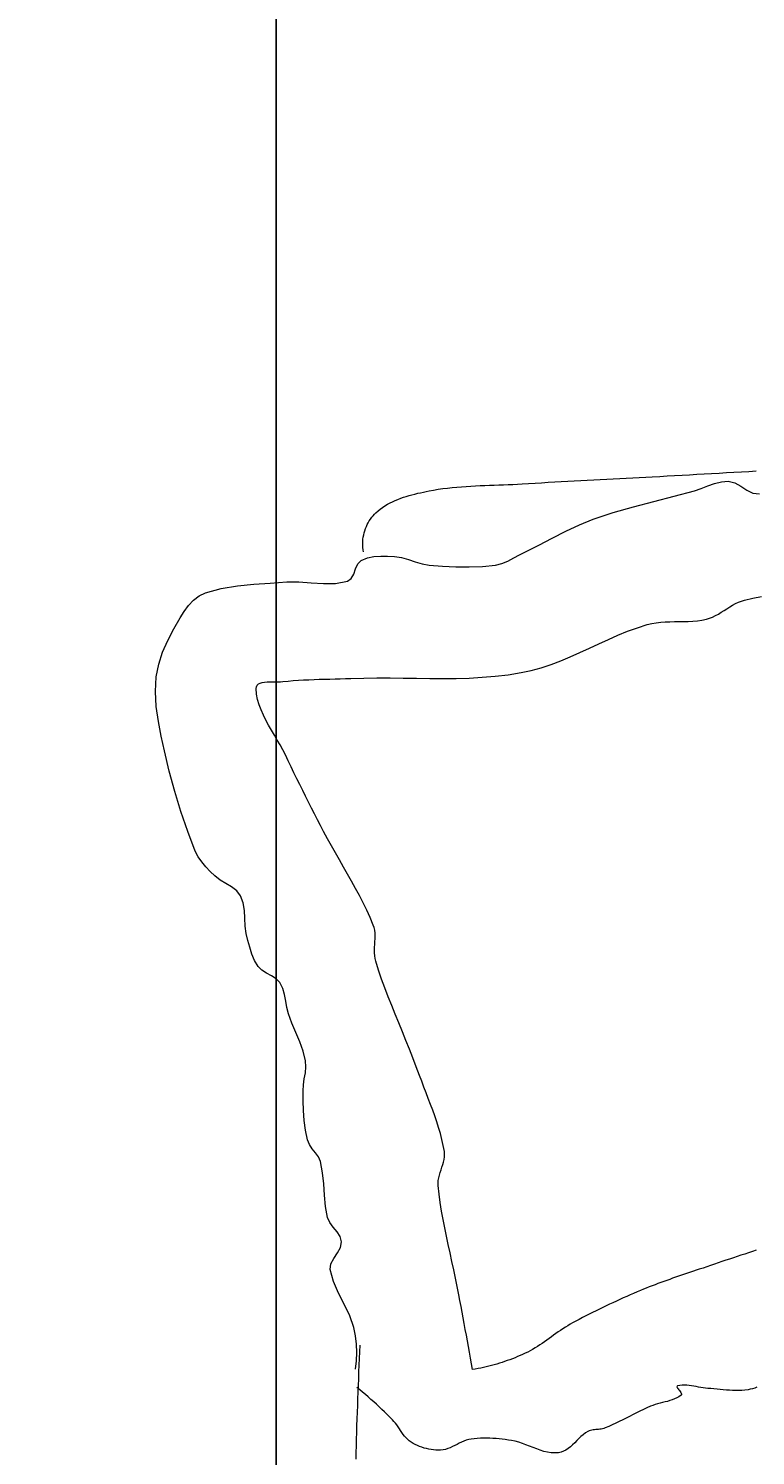
# Model space of a CAD drawing. Units: inches. Extents: x 1770 to 2988, y 1161 to 3221.
# Tile 26 of 44: x 2524 to 2543, y 2330 to 2368. Entities that reach past the tile are written whole.
import ezdxf

# ---------------------------------------------------------------- set-up
doc = ezdxf.new("R2010")
doc.units = ezdxf.units.IN
doc.layers.add('A-ANNO-DIMS', color=2, linetype='Continuous', lineweight=18)
doc.layers.add('A-FURN', color=8, linetype='Continuous', lineweight=13)
doc.styles.get("Standard").update_dxf_attribs({"font": 'arial.ttf'})
doc.dimstyles.get("Standard").update_dxf_attribs({"dimtxt": 0.18, "dimasz": 0.18, "dimexe": 0.18, "dimexo": 0.0625, "dimgap": 0.09, "dimtad": 0, "dimtih": 1, "dimtoh": 1, "dimdec": 4, "dimzin": 0, "dimdsep": 46, "dimtxsty": 'Standard', "dimcen": 0.09, "dimadec": 0, "dimazin": 0, "dimtfac": 1, "dimtdec": 4, "dimtofl": 0, "dimtmove": 0, "dimatfit": 3, "dimfxl": 1, "dimtolj": 1, "dimtzin": 0, "dimarcsym": 0})

# ---------------------------------------------------------------- blocks, each defined once
blk = doc.blocks.new('BED-DOUBLE-PLAN')
for p, q in [((10.769, 99.878), (10.891, 99.883)), ((10.891, 99.883), (11.012, 99.89)), ((11.012, 99.89), (11.134, 99.897)), ((11.134, 99.897), (11.304, 99.907)), ((11.304, 99.907), (11.474, 99.918)), ((11.474, 99.918), (11.644, 99.928)), ((11.644, 99.928), (11.814, 99.938)), ((11.814, 99.938), (11.984, 99.947)), ((11.984, 99.947), (12.154, 99.957)), ((12.154, 99.957), (12.324, 99.966)), ((12.324, 99.966), (12.493, 99.975)), ((12.493, 99.975), (12.663, 99.984)), ((12.663, 99.984), (12.833, 99.993)), ((12.833, 99.993), (13.003, 100.002)), ((13.003, 100.002), (13.173, 100.011)), ((13.173, 100.011), (13.343, 100.019)), ((13.343, 100.019), (13.513, 100.028)), ((13.513, 100.028), (13.683, 100.037)), ((13.683, 100.037), (13.853, 100.046)), ((13.853, 100.046), (14.023, 100.055)), ((14.023, 100.055), (14.193, 100.064)), ((14.193, 100.064), (14.363, 100.073)), ((14.363, 100.073), (14.533, 100.083)), ((14.533, 100.083), (14.727, 100.093)), ((14.727, 100.093), (14.92, 100.104)), ((14.92, 100.104), (15.114, 100.115)), ((15.114, 100.115), (15.308, 100.126)), ((15.308, 100.126), (15.501, 100.137)), ((15.501, 100.137), (15.695, 100.147)), ((15.695, 100.147), (15.888, 100.158)), ((15.888, 100.158), (16.082, 100.169)), ((15.984, 99.845), (16.159, 99.909)), ((16.082, 100.169), (16.276, 100.18)), ((16.159, 99.909), (16.336, 99.954)), ((16.276, 100.18), (16.469, 100.191)), ((16.336, 99.954), (16.516, 99.966)), ((16.469, 100.191), (16.663, 100.202)), ((16.516, 99.966), (16.685, 99.923)), ((16.663, 100.202), (16.857, 100.213)), ((16.685, 99.923), (16.844, 99.835)), ((16.857, 100.213), (17.05, 100.224)), ((17.05, 100.224), (17.244, 100.235)), ((7.892, 99.493), (7.964, 99.52)), ((7.964, 99.52), (8.036, 99.546)), ((8.036, 99.546), (8.109, 99.569)), ((8.109, 99.569), (8.183, 99.591)), ((8.183, 99.591), (8.258, 99.612)), ((8.258, 99.612), (8.332, 99.632)), ((8.332, 99.632), (8.407, 99.65)), ((8.407, 99.65), (8.482, 99.667)), ((8.482, 99.667), (8.556, 99.684)), ((8.556, 99.684), (8.631, 99.699)), ((8.631, 99.699), (8.705, 99.714)), ((8.705, 99.714), (8.824, 99.736)), ((8.824, 99.736), (8.944, 99.756)), ((8.944, 99.756), (9.065, 99.773)), ((9.065, 99.773), (9.185, 99.788)), ((9.185, 99.788), (9.306, 99.802)), ((9.306, 99.802), (9.428, 99.813)), ((9.428, 99.813), (9.549, 99.823)), ((9.549, 99.823), (9.671, 99.831)), ((9.671, 99.831), (9.792, 99.839)), ((9.792, 99.839), (9.914, 99.845)), ((9.914, 99.845), (10.036, 99.851)), ((10.036, 99.851), (10.158, 99.855)), ((10.158, 99.855), (10.28, 99.86)), ((10.28, 99.86), (10.403, 99.864)), ((10.403, 99.864), (10.525, 99.869)), ((10.525, 99.869), (10.647, 99.873)), ((10.647, 99.873), (10.769, 99.878)), ((14.572, 99.437), (15.105, 99.574)), ((15.105, 99.574), (15.635, 99.718)), ((15.635, 99.718), (15.81, 99.777)), ((15.81, 99.777), (15.984, 99.845)), ((16.844, 99.835), (17.001, 99.735)), ((17.001, 99.735), (17.16, 99.657)), ((17.16, 99.657), (17.329, 99.635)), ((7.278, 99.106), (7.316, 99.144)), ((7.316, 99.144), (7.372, 99.193)), ((7.372, 99.193), (7.431, 99.24)), ((7.431, 99.24), (7.491, 99.283)), ((7.491, 99.283), (7.554, 99.324)), ((7.554, 99.324), (7.619, 99.363)), ((7.619, 99.363), (7.685, 99.399)), ((7.685, 99.399), (7.753, 99.432)), ((7.753, 99.432), (7.822, 99.463)), ((7.822, 99.463), (7.892, 99.493)), ((12.992, 98.973), (13.513, 99.145)), ((13.513, 99.145), (14.041, 99.297)), ((14.041, 99.297), (14.572, 99.437)), ((7.046, 98.728), (7.067, 98.781)), ((7.067, 98.781), (7.091, 98.833)), ((7.091, 98.833), (7.117, 98.883)), ((7.117, 98.883), (7.144, 98.931)), ((7.144, 98.931), (7.175, 98.978)), ((7.175, 98.978), (7.207, 99.023)), ((7.207, 99.023), (7.241, 99.066)), ((7.241, 99.066), (7.278, 99.106)), ((12.273, 98.658), (12.628, 98.826)), ((12.628, 98.826), (12.992, 98.973)), ((6.971, 98.342), (6.974, 98.397)), ((6.974, 98.397), (6.979, 98.453)), ((6.979, 98.453), (6.987, 98.509)), ((6.987, 98.509), (6.998, 98.565)), ((6.998, 98.565), (7.012, 98.62)), ((7.012, 98.62), (7.028, 98.674)), ((7.028, 98.674), (7.046, 98.728)), ((11.572, 98.299), (11.922, 98.48)), ((11.922, 98.48), (12.273, 98.658)), ((6.971, 98.287), (6.971, 98.342)), ((6.975, 98.232), (6.971, 98.287)), ((6.981, 98.178), (6.975, 98.232)), ((6.99, 98.125), (6.981, 98.178)), ((10.916, 97.961), (11.066, 98.046)), ((11.066, 98.046), (11.219, 98.125)), ((11.219, 98.125), (11.572, 98.299)), ((6.737, 97.54), (6.785, 97.678)), ((6.785, 97.678), (6.843, 97.807)), ((6.843, 97.807), (6.934, 97.897)), ((6.934, 97.897), (7.094, 97.962)), ((7.094, 97.962), (7.265, 97.998)), ((7.265, 97.998), (7.442, 98.012)), ((7.442, 98.012), (7.621, 98.01)), ((7.621, 98.01), (7.798, 98)), ((7.798, 98), (7.983, 97.971)), ((7.983, 97.971), (8.164, 97.919)), ((8.164, 97.919), (8.344, 97.86)), ((8.344, 97.86), (8.526, 97.807)), ((8.526, 97.807), (8.711, 97.775)), ((8.711, 97.775), (9.057, 97.749)), ((9.057, 97.749), (9.404, 97.731)), ((9.404, 97.731), (9.752, 97.727)), ((9.752, 97.727), (10.099, 97.741)), ((10.099, 97.741), (10.443, 97.776)), ((10.443, 97.776), (10.607, 97.816)), ((10.607, 97.816), (10.764, 97.881)), ((10.764, 97.881), (10.916, 97.961)), ((3.703, 97.235), (4.13, 97.276)), ((4.13, 97.276), (4.56, 97.305)), ((4.56, 97.305), (4.988, 97.334)), ((4.988, 97.334), (5.307, 97.338)), ((5.307, 97.338), (5.628, 97.316)), ((5.628, 97.316), (5.949, 97.294)), ((5.949, 97.294), (6.266, 97.297)), ((6.266, 97.297), (6.576, 97.352)), ((6.576, 97.352), (6.675, 97.422)), ((6.675, 97.422), (6.737, 97.54)), ((2.554, 96.859), (2.703, 96.975)), ((2.703, 96.975), (2.87, 97.055)), ((2.87, 97.055), (3.281, 97.166)), ((3.281, 97.166), (3.703, 97.235)), ((16.942, 96.862), (17.161, 96.913)), ((17.161, 96.913), (17.38, 96.957)), ((2.205, 96.4), (2.307, 96.562)), ((2.307, 96.562), (2.422, 96.718)), ((2.422, 96.718), (2.554, 96.859)), ((16.258, 96.498), (16.332, 96.542)), ((16.332, 96.542), (16.406, 96.589)), ((16.406, 96.589), (16.48, 96.636)), ((16.48, 96.636), (16.554, 96.682)), ((16.554, 96.682), (16.628, 96.726)), ((16.628, 96.726), (16.704, 96.768)), ((16.704, 96.768), (16.781, 96.805)), ((16.781, 96.805), (16.86, 96.837)), ((16.86, 96.837), (16.942, 96.862)), ((2.039, 96.109), (2.205, 96.4)), ((14.142, 96.14), (14.4, 96.222)), ((14.4, 96.222), (14.516, 96.251)), ((14.516, 96.251), (14.632, 96.271)), ((14.632, 96.271), (14.751, 96.284)), ((14.751, 96.284), (14.87, 96.293)), ((14.87, 96.293), (14.99, 96.297)), ((14.99, 96.297), (15.11, 96.299)), ((15.11, 96.299), (15.23, 96.299)), ((15.23, 96.299), (15.351, 96.301)), ((15.351, 96.301), (15.471, 96.304)), ((15.471, 96.304), (15.591, 96.31)), ((15.591, 96.31), (15.71, 96.321)), ((15.71, 96.321), (15.827, 96.338)), ((15.827, 96.338), (15.944, 96.363)), ((15.944, 96.363), (16.026, 96.388)), ((16.026, 96.388), (16.105, 96.419)), ((16.105, 96.419), (16.182, 96.456)), ((16.182, 96.456), (16.258, 96.498)), ((1.749, 95.501), (1.884, 95.809)), ((1.884, 95.809), (2.039, 96.109)), ((13.137, 95.723), (13.385, 95.836)), ((13.385, 95.836), (13.635, 95.945)), ((13.635, 95.945), (13.887, 96.047)), ((13.887, 96.047), (14.142, 96.14)), ((1.646, 95.184), (1.749, 95.501)), ((12.392, 95.383), (12.641, 95.494)), ((12.641, 95.494), (12.889, 95.608)), ((12.889, 95.608), (13.137, 95.723)), ((1.583, 94.858), (1.646, 95.184)), ((11.374, 95.023), (11.633, 95.096)), ((11.633, 95.096), (11.889, 95.182)), ((11.889, 95.182), (12.142, 95.279)), ((12.142, 95.279), (12.392, 95.383)), ((1.562, 94.471), (1.583, 94.858)), ((4.217, 94.64), (4.251, 94.67)), ((4.251, 94.67), (4.296, 94.693)), ((4.296, 94.693), (4.35, 94.708)), ((4.35, 94.708), (4.412, 94.718)), ((4.412, 94.718), (4.479, 94.724)), ((4.479, 94.724), (4.55, 94.727)), ((4.55, 94.727), (4.622, 94.727)), ((4.622, 94.727), (4.693, 94.727)), ((4.693, 94.727), (4.762, 94.727)), ((4.762, 94.727), (4.827, 94.728)), ((4.827, 94.728), (4.886, 94.732)), ((4.886, 94.732), (5.022, 94.746)), ((5.022, 94.746), (5.158, 94.757)), ((5.158, 94.757), (5.294, 94.767)), ((5.294, 94.767), (5.43, 94.775)), ((5.43, 94.775), (5.566, 94.782)), ((5.566, 94.782), (5.703, 94.787)), ((5.703, 94.787), (5.839, 94.792)), ((5.839, 94.792), (5.976, 94.796)), ((5.976, 94.796), (6.112, 94.8)), ((6.112, 94.8), (6.249, 94.804)), ((6.249, 94.804), (6.385, 94.808)), ((6.385, 94.808), (6.522, 94.812)), ((6.522, 94.812), (6.658, 94.817)), ((6.658, 94.817), (7.001, 94.826)), ((7.001, 94.826), (7.344, 94.829)), ((7.344, 94.829), (7.688, 94.827)), ((7.688, 94.827), (8.032, 94.823)), ((8.032, 94.823), (8.376, 94.818)), ((8.376, 94.818), (8.721, 94.814)), ((8.721, 94.814), (9.064, 94.813)), ((9.064, 94.813), (9.408, 94.816)), ((9.408, 94.816), (9.75, 94.826)), ((9.75, 94.826), (10.092, 94.844)), ((10.092, 94.844), (10.433, 94.873)), ((10.433, 94.873), (10.772, 94.913)), ((10.772, 94.913), (11.11, 94.966)), ((11.11, 94.966), (11.374, 95.023)), ((1.584, 94.082), (1.562, 94.471)), ((4.189, 94.55), (4.196, 94.6)), ((4.202, 94.406), (4.189, 94.55)), ((4.196, 94.6), (4.217, 94.64)), ((4.229, 94.265), (4.202, 94.406)), ((1.637, 93.693), (1.584, 94.082)), ((4.269, 94.127), (4.229, 94.265)), ((4.319, 93.992), (4.269, 94.127)), ((4.378, 93.858), (4.319, 93.992)), ((1.711, 93.307), (1.637, 93.693)), ((4.444, 93.726), (4.378, 93.858)), ((4.515, 93.595), (4.444, 93.726)), ((4.59, 93.465), (4.515, 93.595)), ((1.795, 92.924), (1.711, 93.307)), ((4.666, 93.336), (4.59, 93.465)), ((4.742, 93.207), (4.666, 93.336)), ((4.817, 93.077), (4.742, 93.207)), ((1.923, 92.391), (1.795, 92.924)), ((4.888, 92.947), (4.817, 93.077)), ((4.953, 92.816), (4.888, 92.947)), ((5.027, 92.661), (4.953, 92.816)), ((5.102, 92.506), (5.027, 92.661)), ((5.177, 92.351), (5.102, 92.506)), ((2.067, 91.861), (1.923, 92.391)), ((5.252, 92.197), (5.177, 92.351)), ((5.328, 92.043), (5.252, 92.197)), ((2.227, 91.336), (2.067, 91.861)), ((5.405, 91.889), (5.328, 92.043)), ((5.482, 91.736), (5.405, 91.889)), ((5.559, 91.583), (5.482, 91.736)), ((2.405, 90.816), (2.227, 91.336)), ((5.637, 91.43), (5.559, 91.583)), ((5.715, 91.277), (5.637, 91.43)), ((5.794, 91.124), (5.715, 91.277)), ((5.872, 90.971), (5.794, 91.124)), ((5.951, 90.819), (5.872, 90.971)), ((2.601, 90.304), (2.405, 90.816)), ((6.05, 90.63), (5.951, 90.819)), ((6.153, 90.443), (6.05, 90.63)), ((2.675, 90.157), (2.601, 90.304)), ((6.258, 90.258), (6.153, 90.443)), ((6.364, 90.073), (6.258, 90.258)), ((2.769, 90.021), (2.675, 90.157)), ((2.877, 89.894), (2.769, 90.021)), ((2.994, 89.773), (2.877, 89.894)), ((6.47, 89.888), (6.364, 90.073)), ((6.577, 89.703), (6.47, 89.888)), ((3.112, 89.656), (2.994, 89.773)), ((3.247, 89.55), (3.112, 89.656)), ((3.397, 89.459), (3.247, 89.55)), ((3.548, 89.369), (3.397, 89.459)), ((6.682, 89.518), (6.577, 89.703)), ((6.786, 89.331), (6.682, 89.518)), ((3.682, 89.267), (3.548, 89.369)), ((3.785, 89.136), (3.682, 89.267)), ((3.854, 88.952), (3.785, 89.136)), ((6.886, 89.144), (6.786, 89.331)), ((6.984, 88.955), (6.886, 89.144)), ((3.883, 88.756), (3.854, 88.952)), ((3.892, 88.552), (3.883, 88.756)), ((7.077, 88.764), (6.984, 88.955)), ((7.166, 88.571), (7.077, 88.764)), ((3.902, 88.348), (3.892, 88.552)), ((3.933, 88.15), (3.902, 88.348)), ((7.248, 88.375), (7.166, 88.571)), ((7.271, 88.306), (7.248, 88.375)), ((3.976, 87.971), (3.933, 88.15)), ((4.024, 87.792), (3.976, 87.971)), ((7.286, 88.236), (7.271, 88.306)), ((7.294, 88.164), (7.286, 88.236)), ((7.292, 87.942), (7.295, 88.017)), ((7.296, 88.091), (7.294, 88.164)), ((7.295, 88.017), (7.296, 88.091)), ((4.08, 87.617), (4.024, 87.792)), ((4.151, 87.448), (4.08, 87.617)), ((7.28, 87.718), (7.283, 87.792)), ((7.28, 87.644), (7.28, 87.718)), ((7.285, 87.57), (7.28, 87.644)), ((7.283, 87.792), (7.287, 87.867)), ((7.287, 87.867), (7.292, 87.942)), ((4.242, 87.291), (4.151, 87.448)), ((4.34, 87.192), (4.242, 87.291)), ((7.295, 87.498), (7.285, 87.57)), ((7.312, 87.428), (7.295, 87.498)), ((7.387, 87.194), (7.312, 87.428)), ((4.463, 87.117), (4.34, 87.192)), ((4.593, 87.049), (4.463, 87.117)), ((4.715, 86.973), (4.593, 87.049)), ((4.809, 86.872), (4.715, 86.973)), ((4.883, 86.721), (4.809, 86.872)), ((7.467, 86.961), (7.387, 87.194)), ((7.551, 86.73), (7.467, 86.961)), ((4.93, 86.558), (4.883, 86.721)), ((4.962, 86.388), (4.93, 86.558)), ((7.639, 86.501), (7.551, 86.73)), ((7.729, 86.272), (7.639, 86.501)), ((4.993, 86.218), (4.962, 86.388)), ((5.036, 86.052), (4.993, 86.218)), ((7.821, 86.044), (7.729, 86.272)), ((5.126, 85.807), (5.036, 86.052)), ((5.227, 85.565), (5.126, 85.807)), ((7.914, 85.816), (7.821, 86.044)), ((8.007, 85.588), (7.914, 85.816)), ((5.327, 85.323), (5.227, 85.565)), ((8.101, 85.361), (8.007, 85.588)), ((8.193, 85.133), (8.101, 85.361)), ((5.414, 85.077), (5.327, 85.323)), ((5.478, 84.825), (5.414, 85.077)), ((8.284, 84.904), (8.193, 85.133)), ((5.475, 84.513), (5.49, 84.67)), ((5.49, 84.67), (5.478, 84.825)), ((8.372, 84.675), (8.284, 84.904)), ((8.458, 84.444), (8.372, 84.675)), ((5.424, 84.198), (5.448, 84.355)), ((5.448, 84.355), (5.475, 84.513)), ((8.513, 84.293), (8.458, 84.444)), ((8.57, 84.142), (8.513, 84.293)), ((5.415, 84.04), (5.424, 84.198)), ((5.421, 83.783), (5.415, 84.04)), ((8.628, 83.992), (8.57, 84.142)), ((8.685, 83.841), (8.628, 83.992)), ((5.43, 83.526), (5.421, 83.783)), ((5.447, 83.269), (5.43, 83.526)), ((8.743, 83.69), (8.685, 83.841)), ((8.799, 83.539), (8.743, 83.69)), ((8.853, 83.387), (8.799, 83.539)), ((5.478, 83.015), (5.447, 83.269)), ((8.905, 83.235), (8.853, 83.387)), ((8.954, 83.082), (8.905, 83.235)), ((5.528, 82.764), (5.478, 83.015)), ((5.579, 82.643), (5.528, 82.764)), ((8.999, 82.928), (8.954, 83.082)), ((9.039, 82.773), (8.999, 82.928)), ((9.075, 82.617), (9.039, 82.773)), ((5.656, 82.532), (5.579, 82.643)), ((5.743, 82.426), (5.656, 82.532)), ((5.82, 82.316), (5.743, 82.426)), ((9.104, 82.459), (9.075, 82.617)), ((9.111, 82.39), (9.104, 82.459)), ((9.108, 82.322), (9.111, 82.39)), ((5.872, 82.195), (5.82, 82.316)), ((5.926, 81.906), (5.872, 82.195)), ((9.018, 81.98), (9.041, 82.049)), ((9.041, 82.049), (9.064, 82.117)), ((9.064, 82.117), (9.083, 82.185)), ((9.083, 82.185), (9.099, 82.253)), ((9.099, 82.253), (9.108, 82.322)), ((5.953, 81.612), (5.926, 81.906)), ((8.938, 81.637), (8.944, 81.706)), ((8.94, 81.568), (8.938, 81.637)), ((8.944, 81.706), (8.956, 81.775)), ((8.956, 81.775), (8.974, 81.843)), ((8.974, 81.843), (8.995, 81.912)), ((8.995, 81.912), (9.018, 81.98)), ((5.971, 81.317), (5.953, 81.612)), ((5.998, 81.023), (5.971, 81.317)), ((8.966, 81.346), (8.94, 81.568)), ((8.996, 81.125), (8.966, 81.346)), ((6.052, 80.735), (5.998, 81.023)), ((9.032, 80.905), (8.996, 81.125)), ((9.071, 80.685), (9.032, 80.905)), ((6.113, 80.602), (6.052, 80.735)), ((6.204, 80.481), (6.113, 80.602)), ((9.114, 80.465), (9.071, 80.685)), ((6.301, 80.363), (6.204, 80.481)), ((6.381, 80.24), (6.301, 80.363)), ((6.418, 80.104), (6.381, 80.24)), ((9.159, 80.246), (9.114, 80.465)), ((9.205, 80.027), (9.159, 80.246)), ((6.217, 79.668), (6.311, 79.809)), ((6.311, 79.809), (6.39, 79.953)), ((6.39, 79.953), (6.418, 80.104)), ((9.253, 79.809), (9.205, 80.027)), ((9.302, 79.59), (9.253, 79.809)), ((16.946, 79.782), (16.847, 79.75)), ((17.046, 79.814), (16.946, 79.782)), ((17.145, 79.846), (17.046, 79.814)), ((17.245, 79.878), (17.145, 79.846)), ((6.126, 79.375), (6.144, 79.525)), ((6.144, 79.525), (6.217, 79.668)), ((9.349, 79.371), (9.302, 79.59)), ((15.858, 79.416), (15.759, 79.383)), ((15.957, 79.45), (15.858, 79.416)), ((16.055, 79.484), (15.957, 79.45)), ((16.154, 79.517), (16.055, 79.484)), ((16.253, 79.551), (16.154, 79.517)), ((16.352, 79.585), (16.253, 79.551)), ((16.451, 79.618), (16.352, 79.585)), ((16.55, 79.651), (16.451, 79.618)), ((16.649, 79.684), (16.55, 79.651)), ((16.748, 79.717), (16.649, 79.684)), ((16.847, 79.75), (16.748, 79.717)), ((6.207, 79.062), (6.126, 79.375)), ((6.338, 78.762), (6.207, 79.062)), ((9.396, 79.153), (9.349, 79.371)), ((9.441, 78.934), (9.396, 79.153)), ((14.757, 79.037), (14.68, 79.009)), ((14.833, 79.065), (14.757, 79.037)), ((14.91, 79.093), (14.833, 79.065)), ((14.987, 79.12), (14.91, 79.093)), ((15.064, 79.147), (14.987, 79.12)), ((15.141, 79.173), (15.064, 79.147)), ((15.218, 79.2), (15.141, 79.173)), ((15.296, 79.226), (15.218, 79.2)), ((15.373, 79.252), (15.296, 79.226)), ((15.45, 79.278), (15.373, 79.252)), ((15.527, 79.304), (15.45, 79.278)), ((15.605, 79.33), (15.527, 79.304)), ((15.682, 79.356), (15.605, 79.33)), ((15.759, 79.383), (15.682, 79.356)), ((6.489, 78.468), (6.338, 78.762)), ((9.484, 78.714), (9.441, 78.934)), ((9.512, 78.564), (9.484, 78.714)), ((13.865, 78.673), (13.775, 78.633)), ((13.955, 78.713), (13.865, 78.673)), ((14.045, 78.752), (13.955, 78.713)), ((14.135, 78.791), (14.045, 78.752)), ((14.225, 78.83), (14.135, 78.791)), ((14.301, 78.861), (14.225, 78.83)), ((14.376, 78.892), (14.301, 78.861)), ((14.452, 78.922), (14.376, 78.892)), ((14.528, 78.952), (14.452, 78.922)), ((14.604, 78.981), (14.528, 78.952)), ((14.68, 79.009), (14.604, 78.981)), ((6.633, 78.171), (6.489, 78.468)), ((9.54, 78.414), (9.512, 78.564)), ((9.568, 78.264), (9.54, 78.414)), ((13.063, 78.299), (12.974, 78.255)), ((13.151, 78.342), (13.063, 78.299)), ((13.239, 78.385), (13.151, 78.342)), ((13.328, 78.427), (13.239, 78.385)), ((13.417, 78.469), (13.328, 78.427)), ((13.506, 78.511), (13.417, 78.469)), ((13.595, 78.552), (13.506, 78.511)), ((13.685, 78.593), (13.595, 78.552)), ((13.775, 78.633), (13.685, 78.593)), ((6.741, 77.864), (6.633, 78.171)), ((9.596, 78.114), (9.568, 78.264)), ((9.623, 77.964), (9.596, 78.114)), ((9.651, 77.814), (9.623, 77.964)), ((12.324, 77.908), (12.262, 77.869)), ((12.387, 77.946), (12.324, 77.908)), ((12.452, 77.982), (12.387, 77.946)), ((12.538, 78.029), (12.452, 77.982)), ((12.625, 78.075), (12.538, 78.029)), ((12.712, 78.121), (12.625, 78.075)), ((12.799, 78.166), (12.712, 78.121)), ((12.887, 78.211), (12.799, 78.166)), ((12.974, 78.255), (12.887, 78.211)), ((6.786, 77.649), (6.741, 77.864)), ((6.813, 77.43), (6.786, 77.649)), ((9.678, 77.664), (9.651, 77.814)), ((9.706, 77.514), (9.678, 77.664)), ((11.777, 77.532), (11.717, 77.49)), ((11.837, 77.575), (11.777, 77.532)), ((11.897, 77.618), (11.837, 77.575)), ((11.957, 77.661), (11.897, 77.618)), ((12.018, 77.704), (11.957, 77.661)), ((12.078, 77.746), (12.018, 77.704)), ((12.139, 77.788), (12.078, 77.746)), ((12.2, 77.829), (12.139, 77.788)), ((12.262, 77.869), (12.2, 77.829)), ((6.823, 77.209), (6.813, 77.43)), ((6.814, 76.989), (6.823, 77.209)), ((6.89, 77.053), (6.898, 77.228)), ((6.898, 77.228), (6.907, 77.403)), ((9.733, 77.364), (9.706, 77.514)), ((9.76, 77.214), (9.733, 77.364)), ((9.787, 77.064), (9.76, 77.214)), ((11.147, 77.159), (11.082, 77.13)), ((11.213, 77.189), (11.147, 77.159)), ((11.279, 77.221), (11.213, 77.189)), ((11.344, 77.255), (11.279, 77.221)), ((11.408, 77.291), (11.344, 77.255)), ((11.471, 77.328), (11.408, 77.291)), ((11.533, 77.367), (11.471, 77.328)), ((11.595, 77.407), (11.533, 77.367)), ((11.656, 77.448), (11.595, 77.407)), ((11.717, 77.49), (11.656, 77.448)), ((6.788, 76.771), (6.814, 76.989)), ((6.875, 76.702), (6.883, 76.877)), ((6.883, 76.877), (6.89, 77.053)), ((9.814, 76.913), (9.787, 77.064)), ((9.841, 76.763), (9.814, 76.913)), ((9.912, 76.776), (9.841, 76.763)), ((9.982, 76.789), (9.912, 76.776)), ((10.053, 76.803), (9.982, 76.789)), ((10.123, 76.818), (10.053, 76.803)), ((10.194, 76.834), (10.123, 76.818)), ((10.264, 76.851), (10.194, 76.834)), ((10.333, 76.87), (10.264, 76.851)), ((10.403, 76.889), (10.333, 76.87)), ((10.472, 76.909), (10.403, 76.889)), ((10.541, 76.929), (10.472, 76.909)), ((10.61, 76.951), (10.541, 76.929)), ((10.678, 76.974), (10.61, 76.951)), ((10.747, 76.998), (10.678, 76.974)), ((10.814, 77.022), (10.747, 76.998)), ((10.882, 77.048), (10.814, 77.022)), ((10.949, 77.074), (10.882, 77.048)), ((11.015, 77.101), (10.949, 77.074)), ((11.082, 77.13), (11.015, 77.101)), ((6.861, 76.351), (6.868, 76.526)), ((6.868, 76.526), (6.875, 76.702)), ((6.895, 76.236), (6.82, 76.298)), ((6.847, 76), (6.854, 76.176)), ((6.854, 76.176), (6.861, 76.351)), ((6.969, 76.174), (6.895, 76.236)), ((7.042, 76.112), (6.969, 76.174)), ((7.115, 76.049), (7.042, 76.112)), ((7.188, 75.985), (7.115, 76.049)), ((15.229, 76.055), (15.172, 76.024)), ((15.18, 76.329), (15.176, 76.317)), ((15.176, 76.317), (15.18, 76.301)), ((15.194, 76.337), (15.18, 76.329)), ((15.18, 76.301), (15.19, 76.282)), ((15.19, 76.282), (15.205, 76.26)), ((15.253, 76.349), (15.194, 76.337)), ((15.205, 76.26), (15.223, 76.237)), ((15.223, 76.237), (15.242, 76.213)), ((15.282, 76.091), (15.229, 76.055)), ((15.242, 76.213), (15.26, 76.189)), ((15.312, 76.355), (15.253, 76.349)), ((15.26, 76.189), (15.276, 76.166)), ((15.276, 76.166), (15.288, 76.143)), ((15.293, 76.105), (15.282, 76.091)), ((15.288, 76.143), (15.295, 76.123)), ((15.295, 76.123), (15.293, 76.105)), ((15.372, 76.357), (15.312, 76.355)), ((15.432, 76.355), (15.372, 76.357)), ((15.492, 76.349), (15.432, 76.355)), ((15.553, 76.34), (15.492, 76.349)), ((15.614, 76.33), (15.553, 76.34)), ((15.675, 76.319), (15.614, 76.33)), ((15.736, 76.307), (15.675, 76.319)), ((15.797, 76.296), (15.736, 76.307)), ((15.858, 76.286), (15.797, 76.296)), ((15.918, 76.278), (15.858, 76.286)), ((15.979, 76.273), (15.918, 76.278)), ((16.06, 76.268), (15.979, 76.273)), ((16.141, 76.261), (16.06, 76.268)), ((16.222, 76.254), (16.141, 76.261)), ((16.304, 76.246), (16.222, 76.254)), ((16.385, 76.238), (16.304, 76.246)), ((16.466, 76.23), (16.385, 76.238)), ((16.548, 76.224), (16.466, 76.23)), ((16.629, 76.219), (16.548, 76.224)), ((16.71, 76.216), (16.629, 76.219)), ((16.791, 76.216), (16.71, 76.216)), ((16.871, 76.219), (16.791, 76.216)), ((16.952, 76.226), (16.871, 76.219)), ((17.032, 76.237), (16.952, 76.226)), ((17.091, 76.249), (17.032, 76.237)), ((17.149, 76.264), (17.091, 76.249)), ((17.207, 76.282), (17.149, 76.264)), ((17.263, 76.303), (17.207, 76.282)), ((6.835, 75.649), (6.841, 75.825)), ((6.841, 75.825), (6.847, 76)), ((7.26, 75.92), (7.188, 75.985)), ((7.331, 75.856), (7.26, 75.92)), ((7.402, 75.79), (7.331, 75.856)), ((7.472, 75.724), (7.402, 75.79)), ((7.542, 75.657), (7.472, 75.724)), ((7.611, 75.59), (7.542, 75.657)), ((14.21, 75.677), (14.12, 75.632)), ((14.301, 75.72), (14.21, 75.677)), ((14.393, 75.763), (14.301, 75.72)), ((14.485, 75.804), (14.393, 75.763)), ((14.546, 75.828), (14.485, 75.804)), ((14.608, 75.849), (14.546, 75.828)), ((14.671, 75.868), (14.608, 75.849)), ((14.735, 75.885), (14.671, 75.868)), ((14.8, 75.901), (14.735, 75.885)), ((14.864, 75.917), (14.8, 75.901)), ((14.928, 75.934), (14.864, 75.917)), ((14.991, 75.953), (14.928, 75.934)), ((15.053, 75.973), (14.991, 75.953)), ((15.114, 75.997), (15.053, 75.973)), ((15.172, 76.024), (15.114, 75.997)), ((6.818, 75.123), (6.823, 75.298)), ((6.823, 75.298), (6.829, 75.474)), ((6.829, 75.474), (6.835, 75.649)), ((7.68, 75.522), (7.611, 75.59)), ((7.748, 75.454), (7.68, 75.522)), ((7.788, 75.411), (7.748, 75.454)), ((7.826, 75.365), (7.788, 75.411)), ((7.861, 75.318), (7.826, 75.365)), ((7.896, 75.268), (7.861, 75.318)), ((13.487, 75.318), (13.395, 75.277)), ((13.579, 75.361), (13.487, 75.318)), ((13.67, 75.405), (13.579, 75.361)), ((13.76, 75.449), (13.67, 75.405)), ((13.85, 75.495), (13.76, 75.449)), ((13.94, 75.541), (13.85, 75.495)), ((14.03, 75.586), (13.94, 75.541)), ((14.12, 75.632), (14.03, 75.586)), ((6.807, 74.772), (6.812, 74.947)), ((6.812, 74.947), (6.818, 75.123)), ((7.929, 75.219), (7.896, 75.268)), ((7.962, 75.169), (7.929, 75.219)), ((7.996, 75.12), (7.962, 75.169)), ((8.031, 75.071), (7.996, 75.12)), ((8.067, 75.025), (8.031, 75.071)), ((8.105, 74.981), (8.067, 75.025)), ((8.146, 74.939), (8.105, 74.981)), ((8.189, 74.901), (8.146, 74.939)), ((9.676, 74.917), (9.615, 74.894)), ((9.739, 74.935), (9.676, 74.917)), ((9.803, 74.947), (9.739, 74.935)), ((9.883, 74.957), (9.803, 74.947)), ((9.964, 74.964), (9.883, 74.957)), ((10.045, 74.968), (9.964, 74.964)), ((10.126, 74.971), (10.045, 74.968)), ((10.207, 74.971), (10.126, 74.971)), ((10.289, 74.969), (10.207, 74.971)), ((10.37, 74.965), (10.289, 74.969)), ((10.452, 74.96), (10.37, 74.965)), ((10.533, 74.952), (10.452, 74.96)), ((10.614, 74.944), (10.533, 74.952)), ((10.695, 74.934), (10.614, 74.944)), ((10.775, 74.923), (10.695, 74.934)), ((10.856, 74.911), (10.775, 74.923)), ((12.615, 74.961), (12.56, 74.907)), ((12.671, 75.014), (12.615, 74.961)), ((12.728, 75.063), (12.671, 75.014)), ((12.788, 75.107), (12.728, 75.063)), ((12.851, 75.145), (12.788, 75.107)), ((12.883, 75.16), (12.851, 75.145)), ((12.916, 75.171), (12.883, 75.16)), ((12.95, 75.18), (12.916, 75.171)), ((12.985, 75.187), (12.95, 75.18)), ((13.02, 75.192), (12.985, 75.187)), ((13.056, 75.196), (13.02, 75.192)), ((13.092, 75.199), (13.056, 75.196)), ((13.128, 75.202), (13.092, 75.199)), ((13.164, 75.206), (13.128, 75.202)), ((13.199, 75.211), (13.164, 75.206)), ((13.234, 75.218), (13.199, 75.211)), ((13.269, 75.227), (13.234, 75.218)), ((13.302, 75.239), (13.269, 75.227)), ((13.395, 75.277), (13.302, 75.239)), ((6.798, 74.421), (6.803, 74.596)), ((6.803, 74.596), (6.807, 74.772)), ((8.237, 74.868), (8.189, 74.901)), ((8.29, 74.836), (8.237, 74.868)), ((8.344, 74.807), (8.29, 74.836)), ((8.4, 74.78), (8.344, 74.807)), ((8.458, 74.755), (8.4, 74.78)), ((8.516, 74.733), (8.458, 74.755)), ((8.576, 74.714), (8.516, 74.733)), ((8.636, 74.698), (8.576, 74.714)), ((8.697, 74.684), (8.636, 74.698)), ((8.759, 74.673), (8.697, 74.684)), ((8.82, 74.665), (8.759, 74.673)), ((8.882, 74.66), (8.82, 74.665)), ((8.944, 74.658), (8.882, 74.66)), ((9.005, 74.66), (8.944, 74.658)), ((9.07, 74.667), (9.005, 74.66)), ((9.133, 74.68), (9.07, 74.667)), ((9.194, 74.7), (9.133, 74.68)), ((9.255, 74.723), (9.194, 74.7)), ((9.315, 74.75), (9.255, 74.723)), ((9.375, 74.78), (9.315, 74.75)), ((9.435, 74.81), (9.375, 74.78)), ((9.494, 74.84), (9.435, 74.81)), ((9.554, 74.868), (9.494, 74.84)), ((9.615, 74.894), (9.554, 74.868)), ((10.951, 74.892), (10.856, 74.911)), ((11.046, 74.866), (10.951, 74.892)), ((11.14, 74.835), (11.046, 74.866)), ((11.234, 74.8), (11.14, 74.835)), ((11.327, 74.763), (11.234, 74.8)), ((11.421, 74.726), (11.327, 74.763)), ((11.514, 74.69), (11.421, 74.726)), ((11.607, 74.657), (11.514, 74.69)), ((11.7, 74.628), (11.607, 74.657)), ((11.794, 74.605), (11.7, 74.628)), ((11.889, 74.59), (11.794, 74.605)), ((11.984, 74.585), (11.889, 74.59)), ((12.08, 74.59), (11.984, 74.585)), ((12.151, 74.604), (12.08, 74.59)), ((12.217, 74.629), (12.151, 74.604)), ((12.279, 74.662), (12.217, 74.629)), ((12.338, 74.703), (12.279, 74.662)), ((12.396, 74.749), (12.338, 74.703)), ((12.451, 74.799), (12.396, 74.749)), ((12.506, 74.853), (12.451, 74.799)), ((12.56, 74.907), (12.506, 74.853))]:
    blk.add_line(p, q)
blk = doc.blocks.new('*D82')
at = {"layer": 'A-ANNO-DIMS', "color": 0, "lineweight": -2, "transparency": 16777216}
for p, q in [((2443.386, 1610.265), (2443.386, 2570.705)), ((2443.566, 2570.525), (2486.452, 2570.525)), ((2530.124, 2570.525), (2487.238, 2570.525)), ((2530.304, 1610.265), (2530.304, 2570.705))]:
    blk.add_line(p, q, dxfattribs=at)
at = {"layer": 'A-ANNO-DIMS', "color": 0, "transparency": 16777216}
for points in [[(2443.566, 2570.555), (2443.566, 2570.495), (2443.386, 2570.525)], [(2530.124, 2570.555), (2530.124, 2570.495), (2530.304, 2570.525)]]:
    blk.add_solid(points, dxfattribs=at)
at = {"layer": 'Defpoints', "color": 0, "transparency": 16777216}
for p in [(2530.304, 2570.525), (2443.386, 1610.202), (2530.304, 1610.202)]:
    blk.add_point(p, dxfattribs=at)
at = {"layer": 'A-ANNO-DIMS', "color": 0, "transparency": 16777216, "insert": (2486.845, 2570.525), "char_height": 0.18, "attachment_point": 5}
blk.add_mtext('\\A1;86.92', dxfattribs=at)
blk = doc.blocks.new('*D84')
at = {"layer": 'A-ANNO-DIMS', "color": 0, "lineweight": -2, "transparency": 16777216}
for p, q in [((2513.196, 1835.265), (2513.196, 2570.705)), ((2513.376, 2570.525), (2564.56, 2570.525)), ((2616.516, 2570.525), (2565.332, 2570.525)), ((2616.696, 1835.265), (2616.696, 2570.705))]:
    blk.add_line(p, q, dxfattribs=at)
at = {"layer": 'A-ANNO-DIMS', "color": 0, "transparency": 16777216}
for points in [[(2513.376, 2570.555), (2513.376, 2570.495), (2513.196, 2570.525)], [(2616.516, 2570.555), (2616.516, 2570.495), (2616.696, 2570.525)]]:
    blk.add_solid(points, dxfattribs=at)
at = {"layer": 'Defpoints', "color": 0, "transparency": 16777216}
for p in [(2616.696, 2570.525), (2513.196, 1835.202), (2616.696, 1835.202)]:
    blk.add_point(p, dxfattribs=at)
at = {"layer": 'A-ANNO-DIMS', "color": 0, "transparency": 16777216, "insert": (2564.946, 2570.525), "char_height": 0.18, "attachment_point": 5}
blk.add_mtext('\\A1;103.5', dxfattribs=at)

msp = doc.modelspace()

# ---------------------------------------------------------------- block references
at = {"layer": 'A-FURN'}
msp.add_blockref('BED-DOUBLE-PLAN', (2525.5949, 2255.9126), dxfattribs=at)

# ---------------------------------------------------------------- dimensions: what is measured, and where the dimension line sits
at = {"layer": 'A-ANNO-DIMS'}
for base, p1, p2, override, picture, middle in [((2530.3038, 2570.5247), (2443.3863, 1610.2021), (2530.3038, 1610.2021), {"dimdec": 2, "dimlfac": 1, "dimrnd": 0, "dimzin": 0, "dimdsep": 46, "dimlunit": 2}, '*D82', (2486.8451, 2570.5247)), ((2616.696, 2570.5247), (2513.196, 1835.2021), (2616.696, 1835.2021), {"dimdec": 1, "dimlfac": 1, "dimrnd": 0, "dimzin": 0, "dimdsep": 46, "dimlunit": 2}, '*D84', (2564.946, 2570.5247))]:
    dim = msp.add_linear_dim(base=base, p1=p1, p2=p2, dimstyle='Standard', override=override, dxfattribs=at)
    dim.commit()
    dim.dimension.update_dxf_attribs({"geometry": picture, "text_midpoint": middle})

doc.saveas('drawing.dxf')
